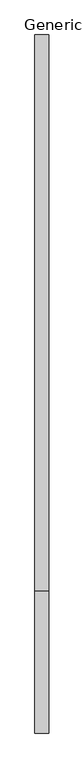
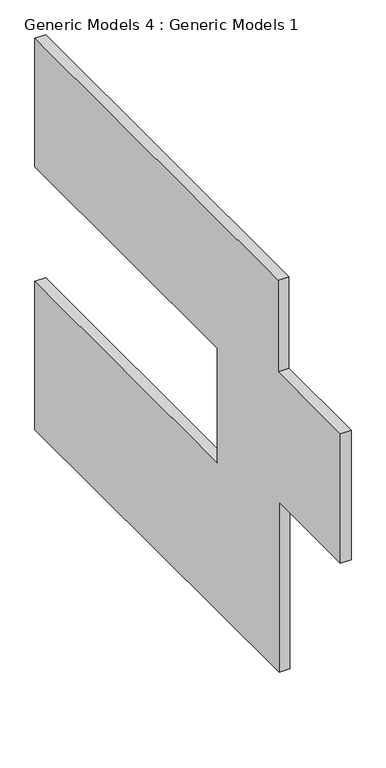
"""IFC4 building model written with IfcOpenShell, lengths in millimetres: proxy geometry, Generic Models 4 : Generic Models 1."""

from ifc_helpers import new_model, si_unit, frame, origin, place, context, project, spatial, polyline, outline, extrude, source, transform, mapped, element, save


def generic_models_4_generic_models_1_d225a6a7(model_context):
    return source(origin(), model_context, "Body", "SweptSolid", [
        extrude(outline(polyline([(-3946.8023495, -2917.9141305), (-3946.8023495, 2214.7139463), (-6979.1363705, 2214.7139463), (-6979.1363705, 6127.75), (-3899.3863708, 6127.75), (-3899.3863708, 8897.2362976), (8140.2136292, 8897.2362976), (8140.2136292, 5015.8429185), (-883.1363705, 5015.8429185), (-883.1363705, 1555.75), (8140.2136292, 1555.75), (8140.2136292, -2917.9141305), (-3946.8023495, -2917.9141305)])), frame((13902.5156363, 0.0, 0.0), z_axis=(1.0, 0.0, 0.0), x_axis=(0.0, 1.0, 0.0)), (0.0, 0.0, 1.0), 304.8),
    ])


if __name__ == "__main__":
    model = new_model("IFC4")
    model_context = context("Model", 3, world=origin())
    ifc_project = project(units=[si_unit("LENGTHUNIT", "METRE", prefix="MILLI")], contexts=[model_context])
    site = spatial("IfcSite", under=ifc_project)
    building = spatial("IfcBuilding", under=site)
    placement = place(None, origin())
    generic_models_4_generic_models_1_shape = generic_models_4_generic_models_1_d225a6a7(model_context)
    element("IfcBuildingElementProxy", 1, Name="Generic Models 4 : Generic Models 1", ObjectType="Generic Models 4 : Generic Models 1", at=placement, inside=building, context=model_context, shape_type="MappedRepresentation", body=[
        mapped(generic_models_4_generic_models_1_shape, transform((0.0, 0.0, 0.0), x_axis=(1.0, 0.0, 0.0), y_axis=(0.0, 1.0, 0.0), z_axis=(0.0, 0.0, 1.0))),
    ])
    save(model, "model.ifc")
